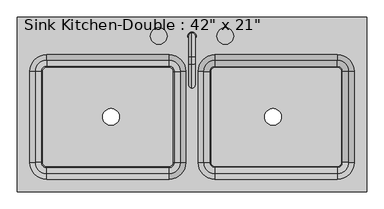
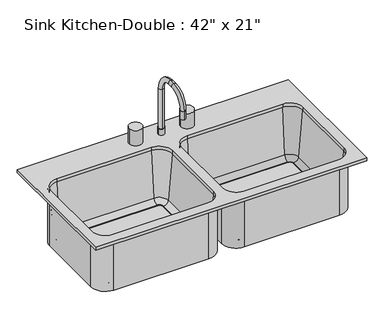
"""IFC4 building model written with IfcOpenShell, lengths in millimetres: flow terminal geometry."""

from ifc_helpers import new_model, si_unit, point, frame, frame_2d, origin, place, context, project, spatial, polyline, circle_curve, ellipse_curve, trimmed, segment, composite_curve, outline, extrude, source, transform, mapped, element, save
from ifc_brep_helpers import plane_surface, cylinder_surface, revolved_surface, advanced_brep


def flow_terminal_a53be723(model_context):
    return source(origin(), model_context, "Body", "SolidModel", [
        advanced_brep(
        [(2.9892406, 211.8954011, 927.1), (28.3892406, 211.8954011, 927.1), (15.6892406, 221.4204011, 1114.425), (15.6892406, 202.3704011, 1114.425), (15.6892406, 202.3704011, 952.5), (15.6892406, 221.4204011, 952.5), (15.6892406, 148.3954011, 1187.45), (15.6892406, 148.3954011, 1168.4), (15.6892406, 126.1704011, 1187.45), (15.6892406, 126.1704011, 1168.4), (15.6892406, 53.1454011, 1114.425), (15.6892406, 72.1954011, 1114.425), (15.6892406, 53.1454011, 1079.5), (15.6892406, 72.1954011, 1079.5), (2.9892406, 211.8954011, 952.5), (28.3892406, 211.8954011, 952.5)],
        [
            (0, 1, circle_curve(frame((15.6892406, 211.8954011, 927.1), z_axis=(0.0, 0.0, -1.0), x_axis=(1.0, 0.0, 0.0)), 12.7)),
            (1, 0, circle_curve(frame((15.6892406, 211.8954011, 927.1), z_axis=(0.0, 0.0, -1.0), x_axis=(1.0, 0.0, 0.0)), 12.7)),
            (2, 3, circle_curve(frame((15.6892406, 211.8954011, 1114.425), z_axis=(0.0, 0.0, -1.0), x_axis=(0.0, -1.0, 0.0)), 9.525)),
            (3, 4),
            (4, 5, circle_curve(frame((15.6892406, 211.8954011, 952.5), z_axis=(0.0, 0.0, 1.0), x_axis=(0.0, -1.0, 0.0)), 9.525)),
            (5, 2),
            (3, 2, circle_curve(frame((15.6892406, 211.8954011, 1114.425), z_axis=(0.0, 0.0, -1.0), x_axis=(0.0, -1.0, 0.0)), 9.525)),
            (5, 4, circle_curve(frame((15.6892406, 211.8954011, 952.5), z_axis=(0.0, 0.0, 1.0), x_axis=(0.0, -1.0, 0.0)), 9.525)),
            (2, 6, circle_curve(frame((15.6892406, 148.3954011, 1114.425), z_axis=(1.0, 0.0, 0.0), x_axis=(0.0, 1.0, 0.0)), 73.025)),
            (6, 7, circle_curve(frame((15.6892406, 148.3954011, 1177.925), z_axis=(0.0, 1.0, 0.0), x_axis=(0.0, 0.0, -1.0)), 9.525)),
            (7, 3, circle_curve(frame((15.6892406, 148.3954011, 1114.425), z_axis=(-1.0, 0.0, 0.0), x_axis=(0.0, 1.0, 0.0)), 53.975)),
            (7, 6, circle_curve(frame((15.6892406, 148.3954011, 1177.925), z_axis=(0.0, 1.0, 0.0), x_axis=(0.0, 0.0, -1.0)), 9.525)),
            (6, 8),
            (8, 9, circle_curve(frame((15.6892406, 126.1704011, 1177.925), z_axis=(0.0, 1.0, 0.0), x_axis=(0.0, 0.0, -1.0)), 9.525)),
            (9, 7),
            (9, 8, circle_curve(frame((15.6892406, 126.1704011, 1177.925), z_axis=(0.0, 1.0, 0.0), x_axis=(0.0, 0.0, -1.0)), 9.525)),
            (8, 10, circle_curve(frame((15.6892406, 126.1704011, 1114.425), z_axis=(1.0, 0.0, 0.0), x_axis=(0.0, 0.0, 1.0)), 73.025)),
            (10, 11, circle_curve(frame((15.6892406, 62.6704011, 1114.425), z_axis=(0.0, 0.0, 1.0), x_axis=(0.0, 1.0, 0.0)), 9.525)),
            (11, 9, circle_curve(frame((15.6892406, 126.1704011, 1114.425), z_axis=(-1.0, 0.0, 0.0), x_axis=(0.0, 0.0, 1.0)), 53.975)),
            (11, 10, circle_curve(frame((15.6892406, 62.6704011, 1114.425), z_axis=(0.0, 0.0, 1.0), x_axis=(0.0, 1.0, 0.0)), 9.525)),
            (12, 13, circle_curve(frame((15.6892406, 62.6704011, 1079.5), z_axis=(0.0, 0.0, -1.0), x_axis=(0.0, 1.0, 0.0)), 9.525)),
            (13, 12, circle_curve(frame((15.6892406, 62.6704011, 1079.5), z_axis=(0.0, 0.0, -1.0), x_axis=(0.0, 1.0, 0.0)), 9.525)),
            (10, 12),
            (13, 11),
            (14, 15, circle_curve(frame((15.6892406, 211.8954011, 952.5), z_axis=(0.0, 0.0, 1.0), x_axis=(1.0, 0.0, 0.0)), 12.7)),
            (15, 14, circle_curve(frame((15.6892406, 211.8954011, 952.5), z_axis=(0.0, 0.0, 1.0), x_axis=(1.0, 0.0, 0.0)), 12.7)),
            (14, 0),
            (1, 15),
        ],
        [
            plane_surface(frame((15.6892406, 202.3704011, 927.1), z_axis=(0.0, 0.0, -1.0), x_axis=(1.0, 0.0, 0.0))),
            cylinder_surface(frame((15.6892406, 211.8954011, 927.1), z_axis=(0.0, 0.0, -1.0), x_axis=(0.0, -1.0, 0.0)), 9.525),
            revolved_surface(trimmed(ellipse_curve(frame((15.6892406, 211.8954011, 1114.425), z_axis=(0.0, 0.0, -1.0), x_axis=(0.0, -1.0, 0.0)), 9.525, 9.525), [point((15.6892406, 221.4204011, 1114.425))], [point((15.6892406, 202.3704011, 1114.425))], True, "CARTESIAN"), (15.6892406, 148.3954011, 1114.425), (1.0, 0.0, 0.0)),
            revolved_surface(trimmed(ellipse_curve(frame((15.6892406, 211.8954011, 1114.425), z_axis=(0.0, 0.0, -1.0), x_axis=(0.0, -1.0, 0.0)), 9.525, 9.525), [point((15.6892406, 202.3704011, 1114.425))], [point((15.6892406, 221.4204011, 1114.425))], True, "CARTESIAN"), (15.6892406, 148.3954011, 1114.425), (1.0, 0.0, 0.0)),
            cylinder_surface(frame((15.6892406, 148.3954011, 1177.925), z_axis=(0.0, 1.0, 0.0), x_axis=(0.0, 0.0, -1.0)), 9.525),
            revolved_surface(trimmed(ellipse_curve(frame((15.6892406, 126.1704011, 1177.925), z_axis=(0.0, 1.0, 0.0), x_axis=(0.0, 0.0, -1.0)), 9.525, 9.525), [point((15.6892406, 126.1704011, 1187.45))], [point((15.6892406, 126.1704011, 1168.4))], True, "CARTESIAN"), (15.6892406, 126.1704011, 1114.425), (1.0, 0.0, 0.0)),
            revolved_surface(trimmed(ellipse_curve(frame((15.6892406, 126.1704011, 1177.925), z_axis=(0.0, 1.0, 0.0), x_axis=(0.0, 0.0, -1.0)), 9.525, 9.525), [point((15.6892406, 126.1704011, 1168.4))], [point((15.6892406, 126.1704011, 1187.45))], True, "CARTESIAN"), (15.6892406, 126.1704011, 1114.425), (1.0, 0.0, 0.0)),
            plane_surface(frame((15.6892406, 53.1454011, 1079.5), z_axis=(0.0, 0.0, -1.0), x_axis=(-1.0, 0.0, 0.0))),
            cylinder_surface(frame((15.6892406, 62.6704011, 1114.425), z_axis=(0.0, 0.0, 1.0), x_axis=(0.0, 1.0, 0.0)), 9.525),
            plane_surface(frame((28.3892406, 211.8954011, 952.5), z_axis=(0.0, 0.0, 1.0), x_axis=(0.0, 1.0, 0.0))),
            cylinder_surface(frame((15.6892406, 211.8954011, 927.1), z_axis=(0.0, 0.0, 1.0), x_axis=(1.0, 0.0, 0.0)), 12.7),
        ],
        [
            (0, [[1, 2]]),
            (1, [[3, 4, 5, 6]]),
            (1, [[7, -6, 8, -4]]),
            (2, [[-3, 9, 10, 11]]),
            (3, [[-7, -11, 12, -9]]),
            (4, [[-10, 13, 14, 15]]),
            (4, [[-12, -15, 16, -13]]),
            (5, [[-14, 17, 18, 19]]),
            (6, [[-16, -19, 20, -17]]),
            (7, [[21, 22]]),
            (8, [[-18, 23, -22, 24]]),
            (8, [[-20, -24, -21, -23]]),
            (9, [[25, 26], [-5, -8]]),
            (10, [[-25, 27, -2, 28]]),
            (10, [[-26, -28, -1, -27]]),
        ],
    ),
        advanced_brep(
        [(549.0892406, 269.0454011, 927.1), (-517.7107594, 269.0454011, 927.1), (-517.7107594, -264.3545989, 927.1), (549.0892406, -264.3545989, 927.1), (-54.1607594, 154.7454011, 927.1), (-3.3607594, 103.9454011, 927.1), (-3.3607594, -175.4545989, 927.1), (-54.1607594, -226.2545989, 927.1), (-428.8107594, -226.2545989, 927.1), (-479.6107594, -175.4545989, 927.1), (-479.6107594, 103.9454011, 927.1), (-428.8107594, 154.7454011, 927.1), (85.5392406, -226.2545989, 927.1), (34.7392406, -175.4545989, 927.1), (34.7392406, 103.9454011, 927.1), (85.5392406, 154.7454011, 927.1), (460.1892406, 154.7454011, 927.1), (510.9892406, 103.9454011, 927.1), (510.9892406, -175.4545989, 927.1), (460.1892406, -226.2545989, 927.1), (549.0892406, 269.0454011, 914.4), (549.0892406, -264.3545989, 914.4), (-517.7107594, -264.3545989, 914.4), (-517.7107594, 269.0454011, 914.4), (85.5392406, 161.0954011, 914.4), (28.3892406, 103.9454011, 914.4), (28.3892406, -175.4545989, 914.4), (85.5392406, -232.6045989, 914.4), (460.1892406, -232.6045989, 914.4), (517.3392406, -175.4545989, 914.4), (517.3392406, 103.9454011, 914.4), (460.1892406, 161.0954011, 914.4), (2.9892406, 103.9454011, 914.4), (-54.1607594, 161.0954011, 914.4), (-428.8107594, 161.0954011, 914.4), (-485.9607594, 103.9454011, 914.4), (-485.9607594, -175.4545989, 914.4), (-428.8107594, -232.6045989, 914.4), (-54.1607594, -232.6045989, 914.4), (2.9892406, -175.4545989, 914.4), (-54.1607594, 154.7454011, 914.4), (-3.3607594, 103.9454011, 914.4), (-3.3607594, -175.4545989, 914.4), (-54.1607594, -226.2545989, 914.4), (-428.8107594, -226.2545989, 914.4), (-479.6107594, -175.4545989, 914.4), (-479.6107594, 103.9454011, 914.4), (-428.8107594, 154.7454011, 914.4), (85.5392406, -226.2545989, 914.4), (34.7392406, -175.4545989, 914.4), (34.7392406, 103.9454011, 914.4), (85.5392406, 154.7454011, 914.4), (460.1892406, 154.7454011, 914.4), (510.9892406, 103.9454011, 914.4), (510.9892406, -175.4545989, 914.4), (460.1892406, -226.2545989, 914.4), (51.2733134, 103.9454011, 725.4146831), (85.5392406, 138.2113283, 725.4146831), (70.2508224, 103.9454011, 708.025), (85.5392406, 119.2338193, 708.025), (72.8392406, 103.9454011, 708.025), (85.5392406, 116.6454011, 708.025), (72.8392406, 103.9454011, 698.5), (85.5392406, 116.6454011, 698.5), (28.3892406, 103.9454011, 698.5), (85.5392406, 161.0954011, 698.5), (51.2733134, -175.4545989, 725.4146831), (70.2508224, -175.4545989, 708.025), (72.8392406, -175.4545989, 708.025), (72.8392406, -175.4545989, 698.5), (28.3892406, -175.4545989, 698.5), (85.5392406, -209.7205261, 725.4146831), (85.5392406, -190.7430171, 708.025), (85.5392406, -188.1545989, 708.025), (85.5392406, -188.1545989, 698.5), (85.5392406, -232.6045989, 698.5), (460.1892406, -209.7205261, 725.4146831), (460.1892406, -190.7430171, 708.025), (460.1892406, -188.1545989, 708.025), (460.1892406, -188.1545989, 698.5), (460.1892406, -232.6045989, 698.5), (494.4551678, -175.4545989, 725.4146831), (475.4776588, -175.4545989, 708.025), (472.8892406, -175.4545989, 708.025), (472.8892406, -175.4545989, 698.5), (517.3392406, -175.4545989, 698.5), (494.4551678, 103.9454011, 725.4146831), (475.4776588, 103.9454011, 708.025), (472.8892406, 103.9454011, 708.025), (472.8892406, 103.9454011, 698.5), (517.3392406, 103.9454011, 698.5), (460.1892406, 138.2113283, 725.4146831), (460.1892406, 119.2338193, 708.025), (460.1892406, 116.6454011, 708.025), (460.1892406, 116.6454011, 698.5), (460.1892406, 161.0954011, 698.5), (2.9892406, 103.9454011, 698.5), (-54.1607594, 161.0954011, 698.5), (-41.4607594, 103.9454011, 698.5), (-54.1607594, 116.6454011, 698.5), (-41.4607594, 103.9454011, 708.025), (-54.1607594, 116.6454011, 708.025), (-38.8723412, 103.9454011, 708.025), (-54.1607594, 119.2338193, 708.025), (-19.8948322, 103.9454011, 725.4146831), (-54.1607594, 138.2113283, 725.4146831), (2.9892406, -175.4545989, 698.5), (-41.4607594, -175.4545989, 698.5), (-41.4607594, -175.4545989, 708.025), (-38.8723412, -175.4545989, 708.025), (-19.8948322, -175.4545989, 725.4146831), (-54.1607594, -232.6045989, 698.5), (-54.1607594, -188.1545989, 698.5), (-54.1607594, -188.1545989, 708.025), (-54.1607594, -190.7430171, 708.025), (-54.1607594, -209.7205261, 725.4146831), (-428.8107594, -232.6045989, 698.5), (-428.8107594, -188.1545989, 698.5), (-428.8107594, -188.1545989, 708.025), (-428.8107594, -190.7430171, 708.025), (-428.8107594, -209.7205261, 725.4146831), (-485.9607594, -175.4545989, 698.5), (-441.5107594, -175.4545989, 698.5), (-441.5107594, -175.4545989, 708.025), (-444.0991776, -175.4545989, 708.025), (-463.0766866, -175.4545989, 725.4146831), (-485.9607594, 103.9454011, 698.5), (-441.5107594, 103.9454011, 698.5), (-441.5107594, 103.9454011, 708.025), (-444.0991776, 103.9454011, 708.025), (-463.0766866, 103.9454011, 725.4146831), (-428.8107594, 161.0954011, 698.5), (-428.8107594, 116.6454011, 698.5), (-428.8107594, 116.6454011, 708.025), (-428.8107594, 119.2338193, 708.025), (-428.8107594, 138.2113283, 725.4146831)],
        [
            (0, 1),
            (1, 2),
            (2, 3),
            (3, 0),
            (4, 5, circle_curve(frame((-54.1607594, 103.9454011, 927.1), z_axis=(0.0, 0.0, -1.0), x_axis=(1.0, 0.0, 0.0)), 50.8)),
            (5, 6),
            (6, 7, circle_curve(frame((-54.1607594, -175.4545989, 927.1), z_axis=(0.0, 0.0, -1.0), x_axis=(1.0, 0.0, 0.0)), 50.8)),
            (7, 8),
            (8, 9, circle_curve(frame((-428.8107594, -175.4545989, 927.1), z_axis=(0.0, 0.0, -1.0), x_axis=(1.0, 0.0, 0.0)), 50.8)),
            (9, 10),
            (10, 11, circle_curve(frame((-428.8107594, 103.9454011, 927.1), z_axis=(0.0, 0.0, -1.0), x_axis=(1.0, 0.0, 0.0)), 50.8)),
            (11, 4),
            (12, 13, circle_curve(frame((85.5392406, -175.4545989, 927.1), z_axis=(0.0, 0.0, -1.0), x_axis=(1.0, 0.0, 0.0)), 50.8)),
            (13, 14),
            (14, 15, circle_curve(frame((85.5392406, 103.9454011, 927.1), z_axis=(0.0, 0.0, -1.0), x_axis=(1.0, 0.0, 0.0)), 50.8)),
            (15, 16),
            (16, 17, circle_curve(frame((460.1892406, 103.9454011, 927.1), z_axis=(0.0, 0.0, -1.0), x_axis=(1.0, 0.0, 0.0)), 50.8)),
            (17, 18),
            (18, 19, circle_curve(frame((460.1892406, -175.4545989, 927.1), z_axis=(0.0, 0.0, -1.0), x_axis=(1.0, 0.0, 0.0)), 50.8)),
            (19, 12),
            (20, 21),
            (21, 22),
            (22, 23),
            (23, 20),
            (24, 25, circle_curve(frame((85.5392406, 103.9454011, 914.4), z_axis=(0.0, 0.0, 1.0), x_axis=(0.0, 1.0, 0.0)), 57.15)),
            (25, 26),
            (26, 27, circle_curve(frame((85.5392406, -175.4545989, 914.4), z_axis=(0.0, 0.0, 1.0), x_axis=(-1.0, 0.0, 0.0)), 57.15)),
            (27, 28),
            (28, 29, circle_curve(frame((460.1892406, -175.4545989, 914.4), z_axis=(0.0, 0.0, 1.0), x_axis=(0.0, -1.0, 0.0)), 57.15)),
            (29, 30),
            (30, 31, circle_curve(frame((460.1892406, 103.9454011, 914.4), z_axis=(0.0, 0.0, 1.0), x_axis=(1.0, 0.0, 0.0)), 57.15)),
            (31, 24),
            (32, 33, circle_curve(frame((-54.1607594, 103.9454011, 914.4), z_axis=(0.0, 0.0, 1.0), x_axis=(0.0, 1.0, 0.0)), 57.15)),
            (33, 34),
            (34, 35, circle_curve(frame((-428.8107594, 103.9454011, 914.4), z_axis=(0.0, 0.0, 1.0), x_axis=(-1.0, 0.0, 0.0)), 57.15)),
            (35, 36),
            (36, 37, circle_curve(frame((-428.8107594, -175.4545989, 914.4), z_axis=(0.0, 0.0, 1.0), x_axis=(0.0, -1.0, 0.0)), 57.15)),
            (37, 38),
            (38, 39, circle_curve(frame((-54.1607594, -175.4545989, 914.4), z_axis=(0.0, 0.0, 1.0), x_axis=(1.0, 0.0, 0.0)), 57.15)),
            (39, 32),
            (0, 20),
            (23, 1),
            (22, 2),
            (21, 3),
            (4, 40),
            (40, 41, circle_curve(frame((-54.1607594, 103.9454011, 914.4), z_axis=(0.0, 0.0, -1.0), x_axis=(1.0, 0.0, 0.0)), 50.8)),
            (41, 5),
            (41, 42),
            (42, 6),
            (42, 43, circle_curve(frame((-54.1607594, -175.4545989, 914.4), z_axis=(0.0, 0.0, -1.0), x_axis=(1.0, 0.0, 0.0)), 50.8)),
            (43, 7),
            (43, 44),
            (44, 8),
            (44, 45, circle_curve(frame((-428.8107594, -175.4545989, 914.4), z_axis=(0.0, 0.0, -1.0), x_axis=(1.0, 0.0, 0.0)), 50.8)),
            (45, 9),
            (45, 46),
            (46, 10),
            (46, 47, circle_curve(frame((-428.8107594, 103.9454011, 914.4), z_axis=(0.0, 0.0, -1.0), x_axis=(1.0, 0.0, 0.0)), 50.8)),
            (47, 11),
            (47, 40),
            (12, 48),
            (48, 49, circle_curve(frame((85.5392406, -175.4545989, 914.4), z_axis=(0.0, 0.0, -1.0), x_axis=(1.0, 0.0, 0.0)), 50.8)),
            (49, 13),
            (49, 50),
            (50, 14),
            (50, 51, circle_curve(frame((85.5392406, 103.9454011, 914.4), z_axis=(0.0, 0.0, -1.0), x_axis=(1.0, 0.0, 0.0)), 50.8)),
            (51, 15),
            (51, 52),
            (52, 16),
            (52, 53, circle_curve(frame((460.1892406, 103.9454011, 914.4), z_axis=(0.0, 0.0, -1.0), x_axis=(1.0, 0.0, 0.0)), 50.8)),
            (53, 17),
            (53, 54),
            (54, 18),
            (54, 55, circle_curve(frame((460.1892406, -175.4545989, 914.4), z_axis=(0.0, 0.0, -1.0), x_axis=(1.0, 0.0, 0.0)), 50.8)),
            (55, 19),
            (55, 48),
            (56, 57, circle_curve(frame((85.5392406, 103.9454011, 725.4146831), z_axis=(0.0, 0.0, -1.0), x_axis=(0.0, 1.0, 0.0)), 34.2659272)),
            (57, 51),
            (50, 56),
            (56, 58, circle_curve(frame((70.2508224, 103.9454011, 727.075), z_axis=(0.0, -1.0, 0.0), x_axis=(1.0, 0.0, 0.0)), 19.05)),
            (58, 59, circle_curve(frame((85.5392406, 103.9454011, 708.025), z_axis=(0.0, 0.0, -1.0), x_axis=(0.0, 1.0, 0.0)), 15.2884182)),
            (59, 57, circle_curve(frame((85.5392406, 119.2338193, 727.075), z_axis=(1.0, 0.0, 0.0), x_axis=(0.0, -1.0, 0.0)), 19.05)),
            (58, 60),
            (60, 61, circle_curve(frame((85.5392406, 103.9454011, 708.025), z_axis=(0.0, 0.0, -1.0), x_axis=(0.0, 1.0, 0.0)), 12.7)),
            (61, 59),
            (60, 62),
            (62, 63, circle_curve(frame((85.5392406, 103.9454011, 698.5), z_axis=(0.0, 0.0, -1.0), x_axis=(0.0, 1.0, 0.0)), 12.7)),
            (63, 61),
            (62, 64),
            (64, 65, circle_curve(frame((85.5392406, 103.9454011, 698.5), z_axis=(0.0, 0.0, -1.0), x_axis=(0.0, 1.0, 0.0)), 57.15)),
            (65, 63),
            (64, 25),
            (24, 65),
            (49, 66),
            (66, 56),
            (66, 67, circle_curve(frame((70.2508224, -175.4545989, 727.075), z_axis=(0.0, -1.0, 0.0), x_axis=(1.0, 0.0, 0.0)), 19.05)),
            (67, 58),
            (67, 68),
            (68, 60),
            (68, 69),
            (69, 62),
            (69, 70),
            (70, 64),
            (70, 26),
            (48, 71),
            (71, 66, circle_curve(frame((85.5392406, -175.4545989, 725.4146831), z_axis=(0.0, 0.0, -1.0), x_axis=(-1.0, 0.0, 0.0)), 34.2659272)),
            (71, 72, circle_curve(frame((85.5392406, -190.7430171, 727.075), z_axis=(1.0, 0.0, 0.0), x_axis=(0.0, 1.0, 0.0)), 19.05)),
            (72, 67, circle_curve(frame((85.5392406, -175.4545989, 708.025), z_axis=(0.0, 0.0, -1.0), x_axis=(-1.0, 0.0, 0.0)), 15.2884182)),
            (72, 73),
            (73, 68, circle_curve(frame((85.5392406, -175.4545989, 708.025), z_axis=(0.0, 0.0, -1.0), x_axis=(-1.0, 0.0, 0.0)), 12.7)),
            (73, 74),
            (74, 69, circle_curve(frame((85.5392406, -175.4545989, 698.5), z_axis=(0.0, 0.0, -1.0), x_axis=(-1.0, 0.0, 0.0)), 12.7)),
            (74, 75),
            (75, 70, circle_curve(frame((85.5392406, -175.4545989, 698.5), z_axis=(0.0, 0.0, -1.0), x_axis=(-1.0, 0.0, 0.0)), 57.15)),
            (75, 27),
            (55, 76),
            (76, 71),
            (76, 77, circle_curve(frame((460.1892406, -190.7430171, 727.075), z_axis=(1.0, 0.0, 0.0), x_axis=(0.0, 1.0, 0.0)), 19.05)),
            (77, 72),
            (77, 78),
            (78, 73),
            (78, 79),
            (79, 74),
            (79, 80),
            (80, 75),
            (80, 28),
            (54, 81),
            (81, 76, circle_curve(frame((460.1892406, -175.4545989, 725.4146831), z_axis=(0.0, 0.0, -1.0), x_axis=(0.0, -1.0, 0.0)), 34.2659272)),
            (81, 82, circle_curve(frame((475.4776588, -175.4545989, 727.075), z_axis=(0.0, 1.0, 0.0), x_axis=(-1.0, 0.0, 0.0)), 19.05)),
            (82, 77, circle_curve(frame((460.1892406, -175.4545989, 708.025), z_axis=(0.0, 0.0, -1.0), x_axis=(0.0, -1.0, 0.0)), 15.2884182)),
            (82, 83),
            (83, 78, circle_curve(frame((460.1892406, -175.4545989, 708.025), z_axis=(0.0, 0.0, -1.0), x_axis=(0.0, -1.0, 0.0)), 12.7)),
            (83, 84),
            (84, 79, circle_curve(frame((460.1892406, -175.4545989, 698.5), z_axis=(0.0, 0.0, -1.0), x_axis=(0.0, -1.0, 0.0)), 12.7)),
            (84, 85),
            (85, 80, circle_curve(frame((460.1892406, -175.4545989, 698.5), z_axis=(0.0, 0.0, -1.0), x_axis=(0.0, -1.0, 0.0)), 57.15)),
            (85, 29),
            (53, 86),
            (86, 81),
            (86, 87, circle_curve(frame((475.4776588, 103.9454011, 727.075), z_axis=(0.0, 1.0, 0.0), x_axis=(-1.0, 0.0, 0.0)), 19.05)),
            (87, 82),
            (87, 88),
            (88, 83),
            (88, 89),
            (89, 84),
            (89, 90),
            (90, 85),
            (90, 30),
            (52, 91),
            (91, 86, circle_curve(frame((460.1892406, 103.9454011, 725.4146831), z_axis=(0.0, 0.0, -1.0), x_axis=(1.0, 0.0, 0.0)), 34.2659272)),
            (91, 92, circle_curve(frame((460.1892406, 119.2338193, 727.075), z_axis=(-1.0, 0.0, 0.0), x_axis=(0.0, -1.0, 0.0)), 19.05)),
            (92, 87, circle_curve(frame((460.1892406, 103.9454011, 708.025), z_axis=(0.0, 0.0, -1.0), x_axis=(1.0, 0.0, 0.0)), 15.2884182)),
            (92, 93),
            (93, 88, circle_curve(frame((460.1892406, 103.9454011, 708.025), z_axis=(0.0, 0.0, -1.0), x_axis=(1.0, 0.0, 0.0)), 12.7)),
            (93, 94),
            (94, 89, circle_curve(frame((460.1892406, 103.9454011, 698.5), z_axis=(0.0, 0.0, -1.0), x_axis=(1.0, 0.0, 0.0)), 12.7)),
            (94, 95),
            (95, 90, circle_curve(frame((460.1892406, 103.9454011, 698.5), z_axis=(0.0, 0.0, -1.0), x_axis=(1.0, 0.0, 0.0)), 57.15)),
            (95, 31),
            (57, 91),
            (59, 92),
            (61, 93),
            (63, 94),
            (65, 95),
            (96, 97, circle_curve(frame((-54.1607594, 103.9454011, 698.5), z_axis=(0.0, 0.0, 1.0), x_axis=(0.0, 1.0, 0.0)), 57.15)),
            (97, 33),
            (32, 96),
            (96, 98),
            (98, 99, circle_curve(frame((-54.1607594, 103.9454011, 698.5), z_axis=(0.0, 0.0, 1.0), x_axis=(0.0, 1.0, 0.0)), 12.7)),
            (99, 97),
            (98, 100),
            (100, 101, circle_curve(frame((-54.1607594, 103.9454011, 708.025), z_axis=(0.0, 0.0, 1.0), x_axis=(0.0, 1.0, 0.0)), 12.7)),
            (101, 99),
            (100, 102),
            (102, 103, circle_curve(frame((-54.1607594, 103.9454011, 708.025), z_axis=(0.0, 0.0, 1.0), x_axis=(0.0, 1.0, 0.0)), 15.2884182)),
            (103, 101),
            (102, 104, circle_curve(frame((-38.8723412, 103.9454011, 727.075), z_axis=(0.0, -1.0, 0.0), x_axis=(1.0, 0.0, 0.0)), 19.05)),
            (104, 105, circle_curve(frame((-54.1607594, 103.9454011, 725.4146831), z_axis=(0.0, 0.0, 1.0), x_axis=(0.0, 1.0, 0.0)), 34.2659272)),
            (105, 103, circle_curve(frame((-54.1607594, 119.2338193, 727.075), z_axis=(-1.0, 0.0, 0.0), x_axis=(0.0, 1.0, 0.0)), 19.05)),
            (104, 41),
            (40, 105),
            (39, 106),
            (106, 96),
            (106, 107),
            (107, 98),
            (107, 108),
            (108, 100),
            (108, 109),
            (109, 102),
            (109, 110, circle_curve(frame((-38.8723412, -175.4545989, 727.075), z_axis=(0.0, -1.0, 0.0), x_axis=(1.0, 0.0, 0.0)), 19.05)),
            (110, 104),
            (110, 42),
            (38, 111),
            (111, 106, circle_curve(frame((-54.1607594, -175.4545989, 698.5), z_axis=(0.0, 0.0, 1.0), x_axis=(1.0, 0.0, 0.0)), 57.15)),
            (111, 112),
            (112, 107, circle_curve(frame((-54.1607594, -175.4545989, 698.5), z_axis=(0.0, 0.0, 1.0), x_axis=(1.0, 0.0, 0.0)), 12.7)),
            (112, 113),
            (113, 108, circle_curve(frame((-54.1607594, -175.4545989, 708.025), z_axis=(0.0, 0.0, 1.0), x_axis=(1.0, 0.0, 0.0)), 12.7)),
            (113, 114),
            (114, 109, circle_curve(frame((-54.1607594, -175.4545989, 708.025), z_axis=(0.0, 0.0, 1.0), x_axis=(1.0, 0.0, 0.0)), 15.2884182)),
            (114, 115, circle_curve(frame((-54.1607594, -190.7430171, 727.075), z_axis=(-1.0, 0.0, 0.0), x_axis=(0.0, -1.0, 0.0)), 19.05)),
            (115, 110, circle_curve(frame((-54.1607594, -175.4545989, 725.4146831), z_axis=(0.0, 0.0, 1.0), x_axis=(1.0, 0.0, 0.0)), 34.2659272)),
            (115, 43),
            (37, 116),
            (116, 111),
            (116, 117),
            (117, 112),
            (117, 118),
            (118, 113),
            (118, 119),
            (119, 114),
            (119, 120, circle_curve(frame((-428.8107594, -190.7430171, 727.075), z_axis=(-1.0, 0.0, 0.0), x_axis=(0.0, -1.0, 0.0)), 19.05)),
            (120, 115),
            (120, 44),
            (36, 121),
            (121, 116, circle_curve(frame((-428.8107594, -175.4545989, 698.5), z_axis=(0.0, 0.0, 1.0), x_axis=(0.0, -1.0, 0.0)), 57.15)),
            (121, 122),
            (122, 117, circle_curve(frame((-428.8107594, -175.4545989, 698.5), z_axis=(0.0, 0.0, 1.0), x_axis=(0.0, -1.0, 0.0)), 12.7)),
            (122, 123),
            (123, 118, circle_curve(frame((-428.8107594, -175.4545989, 708.025), z_axis=(0.0, 0.0, 1.0), x_axis=(0.0, -1.0, 0.0)), 12.7)),
            (123, 124),
            (124, 119, circle_curve(frame((-428.8107594, -175.4545989, 708.025), z_axis=(0.0, 0.0, 1.0), x_axis=(0.0, -1.0, 0.0)), 15.2884182)),
            (124, 125, circle_curve(frame((-444.0991776, -175.4545989, 727.075), z_axis=(0.0, 1.0, 0.0), x_axis=(-1.0, 0.0, 0.0)), 19.05)),
            (125, 120, circle_curve(frame((-428.8107594, -175.4545989, 725.4146831), z_axis=(0.0, 0.0, 1.0), x_axis=(0.0, -1.0, 0.0)), 34.2659272)),
            (125, 45),
            (35, 126),
            (126, 121),
            (126, 127),
            (127, 122),
            (127, 128),
            (128, 123),
            (128, 129),
            (129, 124),
            (129, 130, circle_curve(frame((-444.0991776, 103.9454011, 727.075), z_axis=(0.0, 1.0, 0.0), x_axis=(-1.0, 0.0, 0.0)), 19.05)),
            (130, 125),
            (130, 46),
            (34, 131),
            (131, 126, circle_curve(frame((-428.8107594, 103.9454011, 698.5), z_axis=(0.0, 0.0, 1.0), x_axis=(-1.0, 0.0, 0.0)), 57.15)),
            (131, 132),
            (132, 127, circle_curve(frame((-428.8107594, 103.9454011, 698.5), z_axis=(0.0, 0.0, 1.0), x_axis=(-1.0, 0.0, 0.0)), 12.7)),
            (132, 133),
            (133, 128, circle_curve(frame((-428.8107594, 103.9454011, 708.025), z_axis=(0.0, 0.0, 1.0), x_axis=(-1.0, 0.0, 0.0)), 12.7)),
            (133, 134),
            (134, 129, circle_curve(frame((-428.8107594, 103.9454011, 708.025), z_axis=(0.0, 0.0, 1.0), x_axis=(-1.0, 0.0, 0.0)), 15.2884182)),
            (134, 135, circle_curve(frame((-428.8107594, 119.2338193, 727.075), z_axis=(1.0, 0.0, 0.0), x_axis=(0.0, 1.0, 0.0)), 19.05)),
            (135, 130, circle_curve(frame((-428.8107594, 103.9454011, 725.4146831), z_axis=(0.0, 0.0, 1.0), x_axis=(-1.0, 0.0, 0.0)), 34.2659272)),
            (135, 47),
            (97, 131),
            (99, 132),
            (101, 133),
            (103, 134),
            (105, 135),
        ],
        [
            plane_surface(frame((-517.7107594, 269.0454011, 927.1), z_axis=(0.0, 0.0, 1.0), x_axis=(-1.0, 0.0, 0.0))),
            plane_surface(frame((-517.7107594, 269.0454011, 914.4), z_axis=(0.0, 0.0, -1.0), x_axis=(1.0, 0.0, 0.0))),
            plane_surface(frame((549.0892406, 269.0454011, 927.1), z_axis=(0.0, 1.0, 0.0), x_axis=(0.0, 0.0, -1.0))),
            plane_surface(frame((-517.7107594, 269.0454011, 927.1), z_axis=(-1.0, 0.0, 0.0), x_axis=(0.0, 0.0, -1.0))),
            plane_surface(frame((-517.7107594, -264.3545989, 927.1), z_axis=(0.0, -1.0, 0.0), x_axis=(0.0, 0.0, -1.0))),
            plane_surface(frame((549.0892406, -264.3545989, 927.1), z_axis=(1.0, 0.0, 0.0), x_axis=(0.0, 0.0, -1.0))),
            revolved_surface(polyline([(-3.3607594000000063, 103.9454011, 914.4), (-3.3607594000000063, 103.9454011, 927.1)]), (-54.1607594, 103.9454011, 0.0), (0.0, 0.0, -1.0)),
            plane_surface(frame((-3.3607594, 103.9454011, 927.1), z_axis=(-1.0, 0.0, 0.0), x_axis=(0.0, 0.0, -1.0))),
            revolved_surface(polyline([(-3.3607594000000063, -175.4545989, 914.4), (-3.3607594000000063, -175.4545989, 927.1)]), (-54.1607594, -175.4545989, 0.0), (0.0, 0.0, -1.0)),
            plane_surface(frame((-54.1607594, -226.2545989, 927.1), z_axis=(0.0, 1.0, 0.0), x_axis=(0.0, 0.0, -1.0))),
            revolved_surface(polyline([(-378.0107594, -175.4545989, 914.4), (-378.0107594, -175.4545989, 927.1)]), (-428.8107594, -175.4545989, 0.0), (0.0, 0.0, -1.0)),
            plane_surface(frame((-479.6107594, -175.4545989, 927.1), z_axis=(1.0, 0.0, 0.0), x_axis=(0.0, 0.0, -1.0))),
            revolved_surface(polyline([(-378.0107594, 103.9454011, 914.4), (-378.0107594, 103.9454011, 927.1)]), (-428.8107594, 103.9454011, 0.0), (0.0, 0.0, -1.0)),
            plane_surface(frame((-428.8107594, 154.7454011, 927.1), z_axis=(0.0, -1.0, 0.0), x_axis=(0.0, 0.0, -1.0))),
            revolved_surface(polyline([(136.33924059999998, -175.4545989, 914.4), (136.33924059999998, -175.4545989, 927.1)]), (85.5392406, -175.4545989, 0.0), (0.0, 0.0, -1.0)),
            plane_surface(frame((34.7392406, -175.4545989, 927.1), z_axis=(1.0, 0.0, 0.0), x_axis=(0.0, 0.0, -1.0))),
            revolved_surface(polyline([(136.33924059999998, 103.9454011, 914.4), (136.33924059999998, 103.9454011, 927.1)]), (85.5392406, 103.9454011, 0.0), (0.0, 0.0, -1.0)),
            plane_surface(frame((85.5392406, 154.7454011, 927.1), z_axis=(0.0, -1.0, 0.0), x_axis=(0.0, 0.0, -1.0))),
            revolved_surface(polyline([(510.9892406, 103.9454011, 914.4), (510.9892406, 103.9454011, 927.1)]), (460.1892406, 103.9454011, 0.0), (0.0, 0.0, -1.0)),
            plane_surface(frame((510.9892406, 103.9454011, 927.1), z_axis=(-1.0, 0.0, 0.0), x_axis=(0.0, 0.0, -1.0))),
            revolved_surface(polyline([(510.9892406, -175.4545989, 914.4), (510.9892406, -175.4545989, 927.1)]), (460.1892406, -175.4545989, 0.0), (0.0, 0.0, -1.0)),
            plane_surface(frame((460.1892406, -226.2545989, 927.1), z_axis=(0.0, 1.0, 0.0), x_axis=(0.0, 0.0, -1.0))),
            revolved_surface(polyline([(85.5392406, 154.7454011, 914.4), (85.5392406, 138.2113283, 725.4146831)]), (85.5392406, 103.9454011, 0.0), (0.0, 0.0, 1.0)),
            revolved_surface(trimmed(ellipse_curve(frame((85.5392406, 119.2338193, 727.075), z_axis=(-1.0, 0.0, 0.0), x_axis=(0.0, -1.0, 0.0)), 19.05, 19.05), [point((85.5392406, 138.2113283, 725.4146831))], [point((85.5392406, 119.2338193, 708.025))], True, "CARTESIAN"), (85.5392406, 103.9454011, 0.0), (0.0, 0.0, 1.0)),
            plane_surface(frame((85.5392406, 103.9454011, 708.025), z_axis=(0.0, 0.0, 1.0), x_axis=(0.0, 1.0, 0.0))),
            revolved_surface(polyline([(85.5392406, 116.6454011, 708.025), (85.5392406, 116.6454011, 698.5)]), (85.5392406, 103.9454011, 0.0), (0.0, 0.0, 1.0)),
            plane_surface(frame((85.5392406, 103.9454011, 698.5), z_axis=(0.0, 0.0, -1.0), x_axis=(0.0, 1.0, 0.0))),
            cylinder_surface(frame((85.5392406, 103.9454011, 0.0), z_axis=(0.0, 0.0, 1.0), x_axis=(0.0, 1.0, 0.0)), 57.15),
            plane_surface(frame((34.7392406, 103.9454011, 914.4), z_axis=(0.996194698091745, 0.0, 0.08715574274766508), x_axis=(0.0, -1.0, 0.0))),
            revolved_surface(polyline([(89.3008224, -175.45459889999998, 727.075), (89.3008224, 103.9454011, 727.075)]), (70.2508224, 103.9454011, 727.075), (0.0, -1.0, 0.0)),
            plane_surface(frame((70.2508224, 103.9454011, 708.025), z_axis=(0.0, 0.0, 1.0), x_axis=(0.0, -1.0, 0.0))),
            plane_surface(frame((72.8392406, 103.9454011, 708.025), z_axis=(1.0, 0.0, 0.0), x_axis=(0.0, -1.0, 0.0))),
            plane_surface(frame((72.8392406, 103.9454011, 698.5), z_axis=(0.0, 0.0, -1.0), x_axis=(0.0, -1.0, 0.0))),
            plane_surface(frame((28.3892406, 103.9454011, 698.5), z_axis=(-1.0, 0.0, 0.0), x_axis=(0.0, -1.0, 0.0))),
            revolved_surface(polyline([(34.7392406, -175.4545989, 914.4), (51.2733134, -175.4545989, 725.4146831)]), (85.5392406, -175.4545989, 0.0), (0.0, 0.0, 1.0)),
            revolved_surface(trimmed(ellipse_curve(frame((70.2508224, -175.4545989, 727.075), z_axis=(0.0, -1.0, 0.0), x_axis=(1.0, 0.0, 0.0)), 19.05, 19.05), [point((51.2733134, -175.4545989, 725.4146831))], [point((70.2508224, -175.4545989, 708.025))], True, "CARTESIAN"), (85.5392406, -175.4545989, 0.0), (0.0, 0.0, 1.0)),
            plane_surface(frame((85.5392406, -175.4545989, 708.025), z_axis=(0.0, 0.0, 1.0), x_axis=(-1.0, 0.0, 0.0))),
            revolved_surface(polyline([(72.8392406, -175.4545989, 708.025), (72.8392406, -175.4545989, 698.5)]), (85.5392406, -175.4545989, 0.0), (0.0, 0.0, 1.0)),
            plane_surface(frame((85.5392406, -175.4545989, 698.5), z_axis=(0.0, 0.0, -1.0), x_axis=(-1.0, 0.0, 0.0))),
            cylinder_surface(frame((85.5392406, -175.4545989, 0.0), z_axis=(0.0, 0.0, 1.0), x_axis=(-1.0, 0.0, 0.0)), 57.15),
            plane_surface(frame((85.5392406, -226.2545989, 914.4), z_axis=(0.0, 0.996194698091745, 0.08715574274766508), x_axis=(1.0, 0.0, 0.0))),
            revolved_surface(polyline([(460.18924059999995, -171.6930171, 727.075), (85.5392406, -171.6930171, 727.075)]), (85.5392406, -190.7430171, 727.075), (1.0, 0.0, 0.0)),
            plane_surface(frame((85.5392406, -190.7430171, 708.025), z_axis=(0.0, 0.0, 1.0), x_axis=(1.0, 0.0, 0.0))),
            plane_surface(frame((85.5392406, -188.1545989, 708.025), z_axis=(0.0, 1.0, 0.0), x_axis=(1.0, 0.0, 0.0))),
            plane_surface(frame((85.5392406, -188.1545989, 698.5), z_axis=(0.0, 0.0, -1.0), x_axis=(1.0, 0.0, 0.0))),
            plane_surface(frame((85.5392406, -232.6045989, 698.5), z_axis=(0.0, -1.0, 0.0), x_axis=(1.0, 0.0, 0.0))),
            revolved_surface(polyline([(460.1892406, -226.2545989, 914.4), (460.1892406, -209.7205261, 725.4146831)]), (460.1892406, -175.4545989, 0.0), (0.0, 0.0, 1.0)),
            revolved_surface(trimmed(ellipse_curve(frame((460.1892406, -190.7430171, 727.075), z_axis=(1.0, 0.0, 0.0), x_axis=(0.0, 1.0, 0.0)), 19.05, 19.05), [point((460.1892406, -209.7205261, 725.4146831))], [point((460.1892406, -190.7430171, 708.025))], True, "CARTESIAN"), (460.1892406, -175.4545989, 0.0), (0.0, 0.0, 1.0)),
            plane_surface(frame((460.1892406, -175.4545989, 708.025), z_axis=(0.0, 0.0, 1.0), x_axis=(0.0, -1.0, 0.0))),
            revolved_surface(polyline([(460.1892406, -188.1545989, 708.025), (460.1892406, -188.1545989, 698.5)]), (460.1892406, -175.4545989, 0.0), (0.0, 0.0, 1.0)),
            plane_surface(frame((460.1892406, -175.4545989, 698.5), z_axis=(0.0, 0.0, -1.0), x_axis=(0.0, -1.0, 0.0))),
            cylinder_surface(frame((460.1892406, -175.4545989, 0.0), z_axis=(0.0, 0.0, 1.0), x_axis=(0.0, -1.0, 0.0)), 57.15),
            plane_surface(frame((510.9892406, -175.4545989, 914.4), z_axis=(-0.996194698091745, 0.0, 0.08715574274766508), x_axis=(0.0, 1.0, 0.0))),
            revolved_surface(polyline([(456.42765879999996, 103.94540109999997, 727.075), (456.42765879999996, -175.4545989, 727.075)]), (475.4776588, -175.4545989, 727.075), (0.0, 1.0, 0.0)),
            plane_surface(frame((475.4776588, -175.4545989, 708.025), z_axis=(0.0, 0.0, 1.0), x_axis=(0.0, 1.0, 0.0))),
            plane_surface(frame((472.8892406, -175.4545989, 708.025), z_axis=(-1.0, 0.0, 0.0), x_axis=(0.0, 1.0, 0.0))),
            plane_surface(frame((472.8892406, -175.4545989, 698.5), z_axis=(0.0, 0.0, -1.0), x_axis=(0.0, 1.0, 0.0))),
            plane_surface(frame((517.3392406, -175.4545989, 698.5), z_axis=(1.0, 0.0, 0.0), x_axis=(0.0, 1.0, 0.0))),
            revolved_surface(polyline([(510.9892406, 103.9454011, 914.4), (494.4551678, 103.9454011, 725.4146831)]), (460.1892406, 103.9454011, 0.0), (0.0, 0.0, 1.0)),
            revolved_surface(trimmed(ellipse_curve(frame((475.4776588, 103.9454011, 727.075), z_axis=(0.0, 1.0, 0.0), x_axis=(-1.0, 0.0, 0.0)), 19.05, 19.05), [point((494.4551678, 103.9454011, 725.4146831))], [point((475.4776588, 103.9454011, 708.025))], True, "CARTESIAN"), (460.1892406, 103.9454011, 0.0), (0.0, 0.0, 1.0)),
            plane_surface(frame((460.1892406, 103.9454011, 708.025), z_axis=(0.0, 0.0, 1.0), x_axis=(1.0, 0.0, 0.0))),
            revolved_surface(polyline([(472.8892406, 103.9454011, 708.025), (472.8892406, 103.9454011, 698.5)]), (460.1892406, 103.9454011, 0.0), (0.0, 0.0, 1.0)),
            plane_surface(frame((460.1892406, 103.9454011, 698.5), z_axis=(0.0, 0.0, -1.0), x_axis=(1.0, 0.0, 0.0))),
            cylinder_surface(frame((460.1892406, 103.9454011, 0.0), z_axis=(0.0, 0.0, 1.0), x_axis=(1.0, 0.0, 0.0)), 57.15),
            plane_surface(frame((460.1892406, 154.7454011, 914.4), z_axis=(0.0, -0.996194698091745, 0.08715574274766508), x_axis=(-1.0, 0.0, 0.0))),
            revolved_surface(polyline([(85.53924060000003, 100.1838193, 727.075), (460.1892406, 100.1838193, 727.075)]), (460.1892406, 119.2338193, 727.075), (-1.0, 0.0, 0.0)),
            plane_surface(frame((460.1892406, 119.2338193, 708.025), z_axis=(0.0, 0.0, 1.0), x_axis=(-1.0, 0.0, 0.0))),
            plane_surface(frame((460.1892406, 116.6454011, 708.025), z_axis=(0.0, -1.0, 0.0), x_axis=(-1.0, 0.0, 0.0))),
            plane_surface(frame((460.1892406, 116.6454011, 698.5), z_axis=(0.0, 0.0, -1.0), x_axis=(-1.0, 0.0, 0.0))),
            plane_surface(frame((460.1892406, 161.0954011, 698.5), z_axis=(0.0, 1.0, 0.0), x_axis=(-1.0, 0.0, 0.0))),
            cylinder_surface(frame((-54.1607594, 103.9454011, 0.0), z_axis=(0.0, 0.0, -1.0), x_axis=(0.0, 1.0, 0.0)), 57.15),
            plane_surface(frame((-54.1607594, 103.9454011, 698.5), z_axis=(0.0, 0.0, -1.0), x_axis=(0.0, 1.0, 0.0))),
            revolved_surface(polyline([(-54.1607594, 116.6454011, 698.5), (-54.1607594, 116.6454011, 708.025)]), (-54.1607594, 103.9454011, 0.0), (0.0, 0.0, -1.0)),
            plane_surface(frame((-54.1607594, 103.9454011, 708.025), z_axis=(0.0, 0.0, 1.0), x_axis=(0.0, 1.0, 0.0))),
            revolved_surface(trimmed(ellipse_curve(frame((-54.1607594, 119.2338193, 727.075), z_axis=(1.0, 0.0, 0.0), x_axis=(0.0, 1.0, 0.0)), 19.05, 19.05), [point((-54.1607594, 119.2338193, 708.025))], [point((-54.1607594, 138.2113283, 725.4146831))], True, "CARTESIAN"), (-54.1607594, 103.9454011, 0.0), (0.0, 0.0, -1.0)),
            revolved_surface(polyline([(-54.1607594, 138.2113283, 725.4146831), (-54.1607594, 154.7454011, 914.4)]), (-54.1607594, 103.9454011, 0.0), (0.0, 0.0, -1.0)),
            plane_surface(frame((2.9892406, 103.9454011, 914.4), z_axis=(1.0, 0.0, 0.0), x_axis=(0.0, -1.0, 0.0))),
            plane_surface(frame((2.9892406, 103.9454011, 698.5), z_axis=(0.0, 0.0, -1.0), x_axis=(0.0, -1.0, 0.0))),
            plane_surface(frame((-41.4607594, 103.9454011, 698.5), z_axis=(-1.0, 0.0, 0.0), x_axis=(0.0, -1.0, 0.0))),
            plane_surface(frame((-41.4607594, 103.9454011, 708.025), z_axis=(0.0, 0.0, 1.0), x_axis=(0.0, -1.0, 0.0))),
            revolved_surface(polyline([(-19.8223412, -175.45459889999998, 727.075), (-19.8223412, 103.9454011, 727.075)]), (-38.8723412, 103.9454011, 727.075), (0.0, -1.0, 0.0)),
            plane_surface(frame((-19.8948322, 103.9454011, 725.4146831), z_axis=(-0.9961946980917439, 0.0, 0.08715574274767722), x_axis=(0.0, -1.0, 0.0))),
            cylinder_surface(frame((-54.1607594, -175.4545989, 0.0), z_axis=(0.0, 0.0, -1.0), x_axis=(1.0, 0.0, 0.0)), 57.15),
            plane_surface(frame((-54.1607594, -175.4545989, 698.5), z_axis=(0.0, 0.0, -1.0), x_axis=(1.0, 0.0, 0.0))),
            revolved_surface(polyline([(-41.4607594, -175.4545989, 698.5), (-41.4607594, -175.4545989, 708.025)]), (-54.1607594, -175.4545989, 0.0), (0.0, 0.0, -1.0)),
            plane_surface(frame((-54.1607594, -175.4545989, 708.025), z_axis=(0.0, 0.0, 1.0), x_axis=(1.0, 0.0, 0.0))),
            revolved_surface(trimmed(ellipse_curve(frame((-38.8723412, -175.4545989, 727.075), z_axis=(0.0, -1.0, 0.0), x_axis=(1.0, 0.0, 0.0)), 19.05, 19.05), [point((-38.8723412, -175.4545989, 708.025))], [point((-19.8948322, -175.4545989, 725.4146831))], True, "CARTESIAN"), (-54.1607594, -175.4545989, 0.0), (0.0, 0.0, -1.0)),
            revolved_surface(polyline([(-19.8948322, -175.4545989, 725.4146831), (-3.3607594, -175.4545989, 914.4)]), (-54.1607594, -175.4545989, 0.0), (0.0, 0.0, -1.0)),
            plane_surface(frame((-54.1607594, -232.6045989, 914.4), z_axis=(0.0, -1.0, 0.0), x_axis=(-1.0, 0.0, 0.0))),
            plane_surface(frame((-54.1607594, -232.6045989, 698.5), z_axis=(0.0, 0.0, -1.0), x_axis=(-1.0, 0.0, 0.0))),
            plane_surface(frame((-54.1607594, -188.1545989, 698.5), z_axis=(0.0, 1.0, 0.0), x_axis=(-1.0, 0.0, 0.0))),
            plane_surface(frame((-54.1607594, -188.1545989, 708.025), z_axis=(0.0, 0.0, 1.0), x_axis=(-1.0, 0.0, 0.0))),
            revolved_surface(polyline([(-428.8107594, -209.79301710000001, 727.075), (-54.1607594, -209.79301710000001, 727.075)]), (-54.1607594, -190.7430171, 727.075), (-1.0, 0.0, 0.0)),
            plane_surface(frame((-54.1607594, -209.7205261, 725.4146831), z_axis=(0.0, 0.9961946980917439, 0.08715574274767722), x_axis=(-1.0, 0.0, 0.0))),
            cylinder_surface(frame((-428.8107594, -175.4545989, 0.0), z_axis=(0.0, 0.0, -1.0), x_axis=(0.0, -1.0, 0.0)), 57.15),
            plane_surface(frame((-428.8107594, -175.4545989, 698.5), z_axis=(0.0, 0.0, -1.0), x_axis=(0.0, -1.0, 0.0))),
            revolved_surface(polyline([(-428.8107594, -188.1545989, 698.5), (-428.8107594, -188.1545989, 708.025)]), (-428.8107594, -175.4545989, 0.0), (0.0, 0.0, -1.0)),
            plane_surface(frame((-428.8107594, -175.4545989, 708.025), z_axis=(0.0, 0.0, 1.0), x_axis=(0.0, -1.0, 0.0))),
            revolved_surface(trimmed(ellipse_curve(frame((-428.8107594, -190.7430171, 727.075), z_axis=(-1.0, 0.0, 0.0), x_axis=(0.0, -1.0, 0.0)), 19.05, 19.05), [point((-428.8107594, -190.7430171, 708.025))], [point((-428.8107594, -209.7205261, 725.4146831))], True, "CARTESIAN"), (-428.8107594, -175.4545989, 0.0), (0.0, 0.0, -1.0)),
            revolved_surface(polyline([(-428.8107594, -209.7205261, 725.4146831), (-428.8107594, -226.2545989, 914.4)]), (-428.8107594, -175.4545989, 0.0), (0.0, 0.0, -1.0)),
            plane_surface(frame((-485.9607594, -175.4545989, 914.4), z_axis=(-1.0, 0.0, 0.0), x_axis=(0.0, 1.0, 0.0))),
            plane_surface(frame((-485.9607594, -175.4545989, 698.5), z_axis=(0.0, 0.0, -1.0), x_axis=(0.0, 1.0, 0.0))),
            plane_surface(frame((-441.5107594, -175.4545989, 698.5), z_axis=(1.0, 0.0, 0.0), x_axis=(0.0, 1.0, 0.0))),
            plane_surface(frame((-441.5107594, -175.4545989, 708.025), z_axis=(0.0, 0.0, 1.0), x_axis=(0.0, 1.0, 0.0))),
            revolved_surface(polyline([(-463.14917760000003, 103.94540109999997, 727.075), (-463.14917760000003, -175.4545989, 727.075)]), (-444.0991776, -175.4545989, 727.075), (0.0, 1.0, 0.0)),
            plane_surface(frame((-463.0766866, -175.4545989, 725.4146831), z_axis=(0.9961946980917439, 0.0, 0.08715574274767722), x_axis=(0.0, 1.0, 0.0))),
            cylinder_surface(frame((-428.8107594, 103.9454011, 0.0), z_axis=(0.0, 0.0, -1.0), x_axis=(-1.0, 0.0, 0.0)), 57.15),
            plane_surface(frame((-428.8107594, 103.9454011, 698.5), z_axis=(0.0, 0.0, -1.0), x_axis=(-1.0, 0.0, 0.0))),
            revolved_surface(polyline([(-441.5107594, 103.9454011, 698.5), (-441.5107594, 103.9454011, 708.025)]), (-428.8107594, 103.9454011, 0.0), (0.0, 0.0, -1.0)),
            plane_surface(frame((-428.8107594, 103.9454011, 708.025), z_axis=(0.0, 0.0, 1.0), x_axis=(-1.0, 0.0, 0.0))),
            revolved_surface(trimmed(ellipse_curve(frame((-444.0991776, 103.9454011, 727.075), z_axis=(0.0, 1.0, 0.0), x_axis=(-1.0, 0.0, 0.0)), 19.05, 19.05), [point((-444.0991776, 103.9454011, 708.025))], [point((-463.0766866, 103.9454011, 725.4146831))], True, "CARTESIAN"), (-428.8107594, 103.9454011, 0.0), (0.0, 0.0, -1.0)),
            revolved_surface(polyline([(-463.0766866, 103.9454011, 725.4146831), (-479.6107594, 103.9454011, 914.4)]), (-428.8107594, 103.9454011, 0.0), (0.0, 0.0, -1.0)),
            plane_surface(frame((-428.8107594, 161.0954011, 914.4), z_axis=(0.0, 1.0, 0.0), x_axis=(1.0, 0.0, 0.0))),
            plane_surface(frame((-428.8107594, 161.0954011, 698.5), z_axis=(0.0, 0.0, -1.0), x_axis=(1.0, 0.0, 0.0))),
            plane_surface(frame((-428.8107594, 116.6454011, 698.5), z_axis=(0.0, -1.0, 0.0), x_axis=(1.0, 0.0, 0.0))),
            plane_surface(frame((-428.8107594, 116.6454011, 708.025), z_axis=(0.0, 0.0, 1.0), x_axis=(1.0, 0.0, 0.0))),
            revolved_surface(polyline([(-54.16075940000002, 138.2838193, 727.075), (-428.8107594, 138.2838193, 727.075)]), (-428.8107594, 119.2338193, 727.075), (1.0, 0.0, 0.0)),
            plane_surface(frame((-428.8107594, 138.2113283, 725.4146831), z_axis=(0.0, -0.9961946980917439, 0.08715574274767722), x_axis=(1.0, 0.0, 0.0))),
        ],
        [
            (0, [[1, 2, 3, 4], [5, 6, 7, 8, 9, 10, 11, 12], [13, 14, 15, 16, 17, 18, 19, 20]]),
            (1, [[21, 22, 23, 24], [25, 26, 27, 28, 29, 30, 31, 32], [33, 34, 35, 36, 37, 38, 39, 40]]),
            (2, [[-1, 41, -24, 42]]),
            (3, [[-2, -42, -23, 43]]),
            (4, [[-3, -43, -22, 44]]),
            (5, [[-4, -44, -21, -41]]),
            (6, [[-5, 45, 46, 47]]),
            (7, [[-6, -47, 48, 49]]),
            (8, [[-7, -49, 50, 51]]),
            (9, [[-8, -51, 52, 53]]),
            (10, [[-9, -53, 54, 55]]),
            (11, [[-10, -55, 56, 57]]),
            (12, [[-11, -57, 58, 59]]),
            (13, [[-12, -59, 60, -45]]),
            (14, [[-13, 61, 62, 63]]),
            (15, [[-14, -63, 64, 65]]),
            (16, [[-15, -65, 66, 67]]),
            (17, [[-16, -67, 68, 69]]),
            (18, [[-17, -69, 70, 71]]),
            (19, [[-18, -71, 72, 73]]),
            (20, [[-19, -73, 74, 75]]),
            (21, [[-20, -75, 76, -61]]),
            (22, [[77, 78, -66, 79]]),
            (23, [[-77, 80, 81, 82]]),
            (24, [[-81, 83, 84, 85]]),
            (25, [[-84, 86, 87, 88]]),
            (26, [[-87, 89, 90, 91]]),
            (27, [[-90, 92, -25, 93]]),
            (28, [[-79, -64, 94, 95]]),
            (29, [[-80, -95, 96, 97]]),
            (30, [[-83, -97, 98, 99]]),
            (31, [[-86, -99, 100, 101]]),
            (32, [[-89, -101, 102, 103]]),
            (33, [[-92, -103, 104, -26]]),
            (34, [[-94, -62, 105, 106]]),
            (35, [[-96, -106, 107, 108]]),
            (36, [[-98, -108, 109, 110]]),
            (37, [[-100, -110, 111, 112]]),
            (38, [[-102, -112, 113, 114]]),
            (39, [[-104, -114, 115, -27]]),
            (40, [[-105, -76, 116, 117]]),
            (41, [[-107, -117, 118, 119]]),
            (42, [[-109, -119, 120, 121]]),
            (43, [[-111, -121, 122, 123]]),
            (44, [[-113, -123, 124, 125]]),
            (45, [[-115, -125, 126, -28]]),
            (46, [[-116, -74, 127, 128]]),
            (47, [[-118, -128, 129, 130]]),
            (48, [[-120, -130, 131, 132]]),
            (49, [[-122, -132, 133, 134]]),
            (50, [[-124, -134, 135, 136]]),
            (51, [[-126, -136, 137, -29]]),
            (52, [[-127, -72, 138, 139]]),
            (53, [[-129, -139, 140, 141]]),
            (54, [[-131, -141, 142, 143]]),
            (55, [[-133, -143, 144, 145]]),
            (56, [[-135, -145, 146, 147]]),
            (57, [[-137, -147, 148, -30]]),
            (58, [[-138, -70, 149, 150]]),
            (59, [[-140, -150, 151, 152]]),
            (60, [[-142, -152, 153, 154]]),
            (61, [[-144, -154, 155, 156]]),
            (62, [[-146, -156, 157, 158]]),
            (63, [[-148, -158, 159, -31]]),
            (64, [[-78, 160, -149, -68]]),
            (65, [[-82, 161, -151, -160]]),
            (66, [[-85, 162, -153, -161]]),
            (67, [[-88, 163, -155, -162]]),
            (68, [[-91, 164, -157, -163]]),
            (69, [[-93, -32, -159, -164]]),
            (70, [[165, 166, -33, 167]]),
            (71, [[-165, 168, 169, 170]]),
            (72, [[-169, 171, 172, 173]]),
            (73, [[-172, 174, 175, 176]]),
            (74, [[-175, 177, 178, 179]]),
            (75, [[-178, 180, -46, 181]]),
            (76, [[-167, -40, 182, 183]]),
            (77, [[-168, -183, 184, 185]]),
            (78, [[-171, -185, 186, 187]]),
            (79, [[-174, -187, 188, 189]]),
            (80, [[-177, -189, 190, 191]]),
            (81, [[-180, -191, 192, -48]]),
            (82, [[-182, -39, 193, 194]]),
            (83, [[-184, -194, 195, 196]]),
            (84, [[-186, -196, 197, 198]]),
            (85, [[-188, -198, 199, 200]]),
            (86, [[-190, -200, 201, 202]]),
            (87, [[-192, -202, 203, -50]]),
            (88, [[-193, -38, 204, 205]]),
            (89, [[-195, -205, 206, 207]]),
            (90, [[-197, -207, 208, 209]]),
            (91, [[-199, -209, 210, 211]]),
            (92, [[-201, -211, 212, 213]]),
            (93, [[-203, -213, 214, -52]]),
            (94, [[-204, -37, 215, 216]]),
            (95, [[-206, -216, 217, 218]]),
            (96, [[-208, -218, 219, 220]]),
            (97, [[-210, -220, 221, 222]]),
            (98, [[-212, -222, 223, 224]]),
            (99, [[-214, -224, 225, -54]]),
            (100, [[-215, -36, 226, 227]]),
            (101, [[-217, -227, 228, 229]]),
            (102, [[-219, -229, 230, 231]]),
            (103, [[-221, -231, 232, 233]]),
            (104, [[-223, -233, 234, 235]]),
            (105, [[-225, -235, 236, -56]]),
            (106, [[-226, -35, 237, 238]]),
            (107, [[-228, -238, 239, 240]]),
            (108, [[-230, -240, 241, 242]]),
            (109, [[-232, -242, 243, 244]]),
            (110, [[-234, -244, 245, 246]]),
            (111, [[-236, -246, 247, -58]]),
            (112, [[-166, 248, -237, -34]]),
            (113, [[-170, 249, -239, -248]]),
            (114, [[-173, 250, -241, -249]]),
            (115, [[-176, 251, -243, -250]]),
            (116, [[-179, 252, -245, -251]]),
            (117, [[-181, -60, -247, -252]]),
        ],
    ),
        extrude(outline(composite_curve([segment(trimmed(circle_curve(frame_2d((460.1892406, 106.5338193)), 12.7), [point((460.1892406, 119.2338193))], [point((472.8892406, 106.5338193))], False, "CARTESIAN"), True, "CONTINUOUS"), segment(polyline([(472.8892406, 106.5338193), (472.8892406, -175.4545989)]), True, "CONTINUOUS"), segment(trimmed(circle_curve(frame_2d((460.1892406, -175.4545989)), 12.7), [point((472.8892406, -175.4545989))], [point((460.1892406, -188.1545989))], False, "CARTESIAN"), True, "CONTINUOUS"), segment(polyline([(460.1892406, -188.1545989), (85.5392406, -188.1545989)]), True, "CONTINUOUS"), segment(trimmed(circle_curve(frame_2d((85.5392406, -175.4545989)), 12.7), [point((85.5392406, -188.1545989))], [point((72.8392406, -175.4545989))], False, "CARTESIAN"), True, "CONTINUOUS"), segment(polyline([(72.8392406, -175.4545989), (72.8392406, 106.5338193)]), True, "CONTINUOUS"), segment(trimmed(circle_curve(frame_2d((85.5392406, 106.5338193)), 12.7), [point((72.8392406, 106.5338193))], [point((85.5392406, 119.2338193))], False, "CARTESIAN"), True, "CONTINUOUS"), segment(polyline([(85.5392406, 119.2338193), (460.1892406, 119.2338193)]), True, "CONTINUOUS")], self_intersect=False), holes=[composite_curve([segment(trimmed(circle_curve(frame_2d((263.3392406, -35.7545989)), 25.4), [point((237.9392406, -35.7545989))], [point((288.7392406, -35.7545989))], True, "CARTESIAN"), True, "CONTINUOUS"), segment(trimmed(circle_curve(frame_2d((263.3392406, -35.7545989)), 25.4), [point((288.7392406, -35.7545989))], [point((237.9392406, -35.7545989))], True, "CARTESIAN"), True, "CONTINUOUS")], self_intersect=False)]), frame((0.0, 0.0, 698.5), z_axis=(0.0, 0.0, 1.0), x_axis=(1.0, 0.0, 0.0)), (0.0, 0.0, 1.0), 9.525),
        extrude(outline(composite_curve([segment(trimmed(circle_curve(frame_2d((-85.9107594, 211.8954011)), 25.4), [point((-111.3107594, 211.8954011))], [point((-60.5107594, 211.8954011))], False, "CARTESIAN"), True, "CONTINUOUS"), segment(trimmed(circle_curve(frame_2d((-85.9107594, 211.8954011)), 25.4), [point((-60.5107594, 211.8954011))], [point((-111.3107594, 211.8954011))], False, "CARTESIAN"), True, "CONTINUOUS")], self_intersect=False)), frame((0.0, 0.0, 927.1), z_axis=(0.0, 0.0, 1.0), x_axis=(1.0, 0.0, 0.0)), (0.0, 0.0, 1.0), 63.5),
        extrude(outline(composite_curve([segment(trimmed(circle_curve(frame_2d((117.2892406, 211.8954011)), 25.4), [point((91.8892406, 211.8954011))], [point((142.6892406, 211.8954011))], False, "CARTESIAN"), True, "CONTINUOUS"), segment(trimmed(circle_curve(frame_2d((117.2892406, 211.8954011)), 25.4), [point((142.6892406, 211.8954011))], [point((91.8892406, 211.8954011))], False, "CARTESIAN"), True, "CONTINUOUS")], self_intersect=False)), frame((0.0, 0.0, 927.1), z_axis=(0.0, 0.0, 1.0), x_axis=(1.0, 0.0, 0.0)), (0.0, 0.0, 1.0), 63.5),
        extrude(outline(composite_curve([segment(trimmed(circle_curve(frame_2d((-54.1607594, 103.9454011)), 12.7), [point((-54.1607594, 116.6454011))], [point((-41.4607594, 103.9454011))], False, "CARTESIAN"), True, "CONTINUOUS"), segment(polyline([(-41.4607594, 103.9454011), (-41.4607594, -175.4545989)]), True, "CONTINUOUS"), segment(trimmed(circle_curve(frame_2d((-54.1607594, -175.4545989)), 12.7), [point((-41.4607594, -175.4545989))], [point((-54.1607594, -188.1545989))], False, "CARTESIAN"), True, "CONTINUOUS"), segment(polyline([(-54.1607594, -188.1545989), (-428.8107594, -188.1545989)]), True, "CONTINUOUS"), segment(trimmed(circle_curve(frame_2d((-428.8107594, -175.4545989)), 12.7), [point((-428.8107594, -188.1545989))], [point((-441.5107594, -175.4545989))], False, "CARTESIAN"), True, "CONTINUOUS"), segment(polyline([(-441.5107594, -175.4545989), (-441.5107594, 103.9454011)]), True, "CONTINUOUS"), segment(trimmed(circle_curve(frame_2d((-428.8107594, 103.9454011)), 12.7), [point((-441.5107594, 103.9454011))], [point((-428.8107594, 116.6454011))], False, "CARTESIAN"), True, "CONTINUOUS"), segment(polyline([(-428.8107594, 116.6454011), (-54.1607594, 116.6454011)]), True, "CONTINUOUS")], self_intersect=False), holes=[composite_curve([segment(trimmed(circle_curve(frame_2d((-231.9607594, -35.7545989)), 25.4), [point((-257.3607594, -35.7545989))], [point((-206.5607594, -35.7545989))], True, "CARTESIAN"), True, "CONTINUOUS"), segment(trimmed(circle_curve(frame_2d((-231.9607594, -35.7545989)), 25.4), [point((-206.5607594, -35.7545989))], [point((-257.3607594, -35.7545989))], True, "CARTESIAN"), True, "CONTINUOUS")], self_intersect=False)]), frame((0.0, 0.0, 698.5), z_axis=(0.0, 0.0, 1.0), x_axis=(1.0, 0.0, 0.0)), (0.0, 0.0, 1.0), 9.525),
    ])


if __name__ == "__main__":
    model = new_model("IFC4")
    model_context = context("Model", 3, world=origin())
    ifc_project = project(units=[si_unit("LENGTHUNIT", "METRE", prefix="MILLI")], contexts=[model_context])
    site = spatial("IfcSite", under=ifc_project)
    building = spatial("IfcBuilding", under=site)
    placement = place(None, origin())
    flow_terminal_shape = flow_terminal_a53be723(model_context)
    element("IfcFlowTerminal", 1, ObjectType="Sink Kitchen-Double : 42\" x 21\"", at=placement, inside=building, context=model_context, shape_type="MappedRepresentation", body=[
        mapped(flow_terminal_shape, transform((0.0, 0.0, 0.0), x_axis=(1.0, 0.0, 0.0), y_axis=(0.0, 1.0, 0.0), z_axis=(0.0, 0.0, 1.0))),
    ])
    save(model, "model.ifc")

# Revit data of these elements
# Type "Sink Kitchen-Double : 42\" x 21\""
#   Assembly Code = "D2010410"
#   Counter Height = 3' - 0"
#   Depth = 1' - 9"
#   Width = 3' - 6"
#   Faucet Material = Steel, Polished
#   Sink Material = Steel, Polished
#   Default Elevation = 0
# Element 1 (IfcFlowTerminal, "Sink Kitchen-Double : 42\" x 21\"")
#   Materials on its faces: "Steel, Polished"
# Materials
#   "Steel, Polished": class "Metal", colour RGB 57 57 57, transparency 0, Description = "Polished steel", Cost = 0
